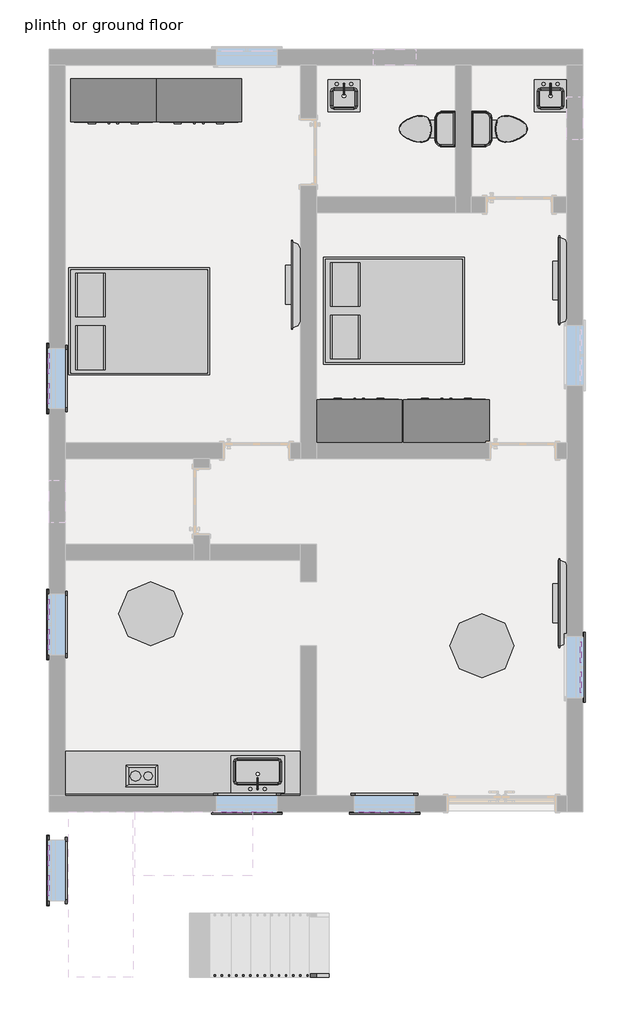
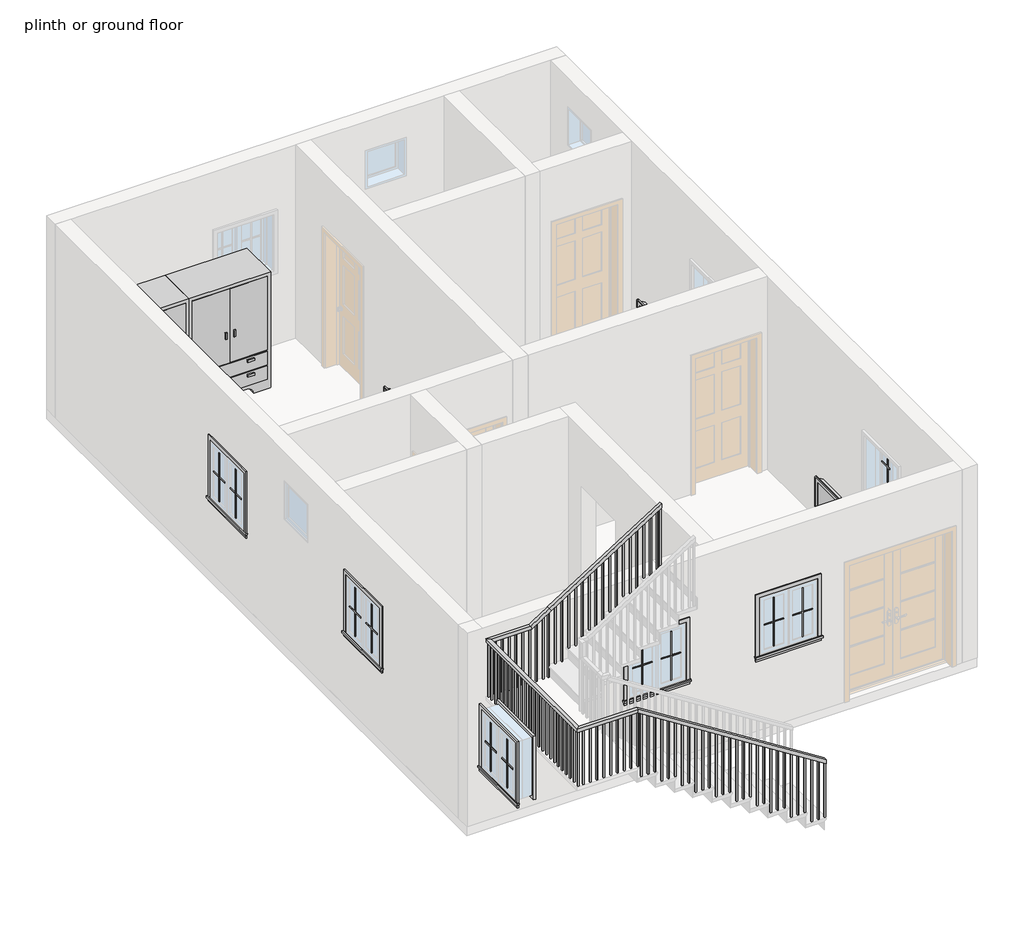
# One storey, part 2 of 3: 24 proxies, 12 furniture elements, 5 flow terminals, 1 railing.
"""IFC4 building model written with IfcOpenShell, lengths in millimetres."""

from ifc_helpers import new_model, si_unit, frame, origin, place, context, project, spatial, polyline, outline, extrude, faceted_brep, transform, mapped, element, save
from components import proxy_fb8a77b2, muntin_pattern_2x2_muntin_pattern_2x2_b3fe6957, muntin_pattern_2x2_muntin_pattern_2x2_3e0ecaf2, trim_window_exterior_flat_with_sill_41619996, trim_window_interior_flat_picture_frame_51c85655, flow_terminal_2ed30f95, flow_terminal_4d548711, toilet_domestic_3d_toilet_domestic_3d_ba6479b0, toilet_domestic_3d_toilet_domestic_3d_30431060, furniture_0315470b, furniture_691b2c5f, furniture_0b81fedb, furniture_ec754799, furniture_52f35bf4, furniture_82e269c4

model = new_model("IFC4")

# Units and contexts
model_context = context("Model", 3, world=origin())
ifc_project = project(units=[si_unit("LENGTHUNIT", "METRE", prefix="MILLI")], contexts=[model_context])

# Site, building, storey
site = spatial("IfcSite", under=ifc_project)
building = spatial("IfcBuilding", under=site)
storey = spatial("IfcBuildingStorey", under=building, Name="plinth or ground floor", Elevation=609.6)

# Proxies
placement = place(None, origin())
proxy_shape = proxy_fb8a77b2(model_context)
element("IfcBuildingElementProxy", 1, Name="Cook Top-2 Unit : 12\" x 18\"", ObjectType="Cook Top-2 Unit : 12\" x 18\"", at=placement, inside=storey, context=model_context, shape_type="MappedRepresentation", body=[
    mapped(proxy_shape, transform((20364.3384757, 6764.8409313, 609.6), x_axis=(0.0, 1.0, 0.0), y_axis=(-1.0, 0.0, 0.0), z_axis=(0.0, 0.0, 1.0))),
])
muntin_pattern_2x2_muntin_pattern_2x2_shape = muntin_pattern_2x2_muntin_pattern_2x2_b3fe6957(model_context)
element("IfcBuildingElementProxy", 2, Name="Muntin Pattern_2x2 : Muntin Pattern_2x2", ObjectType="Muntin Pattern_2x2 : Muntin Pattern_2x2", at=placement, inside=storey, context=model_context, shape_type="MappedRepresentation", body=[
    mapped(muntin_pattern_2x2_muntin_pattern_2x2_shape, transform((19022.8386801, 8785.7284313, 1863.725), x_axis=(0.0, 1.0, 0.0), y_axis=(-1.0, 0.0, 0.0), z_axis=(0.0, 0.0, 1.0))),
])
element("IfcBuildingElementProxy", 3, Name="Muntin Pattern_2x2 : Muntin Pattern_2x2", ObjectType="Muntin Pattern_2x2 : Muntin Pattern_2x2", at=placement, inside=storey, context=model_context, shape_type="MappedRepresentation", body=[
    mapped(muntin_pattern_2x2_muntin_pattern_2x2_shape, transform((19022.8386801, 12290.9284313, 1863.725), x_axis=(0.0, 1.0, 0.0), y_axis=(-1.0, 0.0, 0.0), z_axis=(0.0, 0.0, 1.0))),
])
element("IfcBuildingElementProxy", 4, Name="Muntin Pattern_2x2 : Muntin Pattern_2x2", ObjectType="Muntin Pattern_2x2 : Muntin Pattern_2x2", at=placement, inside=storey, context=model_context, shape_type="MappedRepresentation", body=[
    mapped(muntin_pattern_2x2_muntin_pattern_2x2_shape, transform((26611.0886801, 8604.7534313, 1863.725), x_axis=(0.0, -1.0, 0.0), y_axis=(1.0, 0.0, 0.0), z_axis=(0.0, 0.0, 1.0))),
])
element("IfcBuildingElementProxy", 5, Name="Muntin Pattern_2x2 : Muntin Pattern_2x2", ObjectType="Muntin Pattern_2x2 : Muntin Pattern_2x2", at=placement, inside=storey, context=model_context, shape_type="MappedRepresentation", body=[
    mapped(muntin_pattern_2x2_muntin_pattern_2x2_shape, transform((22047.0261801, 6342.5659313, 1863.725), x_axis=(-1.0, 0.0, 0.0), y_axis=(0.0, -1.0, 0.0), z_axis=(0.0, 0.0, 1.0))),
])
element("IfcBuildingElementProxy", 6, Name="Muntin Pattern_2x2 : Muntin Pattern_2x2", ObjectType="Muntin Pattern_2x2 : Muntin Pattern_2x2", at=placement, inside=storey, context=model_context, shape_type="MappedRepresentation", body=[
    mapped(muntin_pattern_2x2_muntin_pattern_2x2_shape, transform((24009.1761801, 6342.5659313, 1863.725), x_axis=(-1.0, 0.0, 0.0), y_axis=(0.0, -1.0, 0.0), z_axis=(0.0, 0.0, 1.0))),
])
element("IfcBuildingElementProxy", 7, Name="Muntin Pattern_2x2 : Muntin Pattern_2x2", ObjectType="Muntin Pattern_2x2 : Muntin Pattern_2x2", at=placement, inside=storey, context=model_context, shape_type="MappedRepresentation", body=[
    mapped(muntin_pattern_2x2_muntin_pattern_2x2_shape, transform((19022.8386801, 5280.5284313, 1863.725), x_axis=(0.0, 1.0, 0.0), y_axis=(-1.0, 0.0, 0.0), z_axis=(0.0, 0.0, 1.0))),
])
muntin_pattern_2x2_muntin_pattern_2x2_2_shape = muntin_pattern_2x2_muntin_pattern_2x2_3e0ecaf2(model_context)
element("IfcBuildingElementProxy", 8, Name="Muntin Pattern_2x2 : Muntin Pattern_2x2", ObjectType="Muntin Pattern_2x2 : Muntin Pattern_2x2", at=placement, inside=storey, context=model_context, shape_type="MappedRepresentation", body=[
    mapped(muntin_pattern_2x2_muntin_pattern_2x2_2_shape, transform((19022.8386801, 9214.3534313, 1863.725), x_axis=(0.0, -1.0, 0.0), y_axis=(1.0, 0.0, 0.0), z_axis=(0.0, 0.0, 1.0))),
])
element("IfcBuildingElementProxy", 9, Name="Muntin Pattern_2x2 : Muntin Pattern_2x2", ObjectType="Muntin Pattern_2x2 : Muntin Pattern_2x2", at=placement, inside=storey, context=model_context, shape_type="MappedRepresentation", body=[
    mapped(muntin_pattern_2x2_muntin_pattern_2x2_2_shape, transform((19022.8386801, 12719.5534313, 1863.725), x_axis=(0.0, -1.0, 0.0), y_axis=(1.0, 0.0, 0.0), z_axis=(0.0, 0.0, 1.0))),
])
element("IfcBuildingElementProxy", 10, Name="Muntin Pattern_2x2 : Muntin Pattern_2x2", ObjectType="Muntin Pattern_2x2 : Muntin Pattern_2x2", at=placement, inside=storey, context=model_context, shape_type="MappedRepresentation", body=[
    mapped(muntin_pattern_2x2_muntin_pattern_2x2_2_shape, transform((26611.0886801, 8176.1284313, 1863.725), x_axis=(0.0, 1.0, 0.0), y_axis=(-1.0, 0.0, 0.0), z_axis=(0.0, 0.0, 1.0))),
])
element("IfcBuildingElementProxy", 11, Name="Muntin Pattern_2x2 : Muntin Pattern_2x2", ObjectType="Muntin Pattern_2x2 : Muntin Pattern_2x2", at=placement, inside=storey, context=model_context, shape_type="MappedRepresentation", body=[
    mapped(muntin_pattern_2x2_muntin_pattern_2x2_2_shape, transform((21618.4011801, 6342.5659313, 1863.725), x_axis=(1.0, 0.0, 0.0), y_axis=(0.0, 1.0, 0.0), z_axis=(0.0, 0.0, 1.0))),
])
element("IfcBuildingElementProxy", 12, Name="Muntin Pattern_2x2 : Muntin Pattern_2x2", ObjectType="Muntin Pattern_2x2 : Muntin Pattern_2x2", at=placement, inside=storey, context=model_context, shape_type="MappedRepresentation", body=[
    mapped(muntin_pattern_2x2_muntin_pattern_2x2_2_shape, transform((23580.5511801, 6342.5659313, 1863.725), x_axis=(1.0, 0.0, 0.0), y_axis=(0.0, 1.0, 0.0), z_axis=(0.0, 0.0, 1.0))),
])
element("IfcBuildingElementProxy", 13, Name="Muntin Pattern_2x2 : Muntin Pattern_2x2", ObjectType="Muntin Pattern_2x2 : Muntin Pattern_2x2", at=placement, inside=storey, context=model_context, shape_type="MappedRepresentation", body=[
    mapped(muntin_pattern_2x2_muntin_pattern_2x2_2_shape, transform((19022.8386801, 5709.1534313, 1863.725), x_axis=(0.0, -1.0, 0.0), y_axis=(1.0, 0.0, 0.0), z_axis=(0.0, 0.0, 1.0))),
])
trim_window_exterior_flat_with_sill_shape = trim_window_exterior_flat_with_sill_41619996(model_context)
element("IfcBuildingElementProxy", 14, Name="Trim-Window-Exterior-Flat : with Sill", ObjectType="Trim-Window-Exterior-Flat : with Sill", at=placement, inside=storey, context=model_context, shape_type="MappedRepresentation", body=[
    mapped(trim_window_exterior_flat_with_sill_shape, transform((19013.3136801, 9000.0409313, 2708.275), x_axis=(0.0, -1.0, 0.0), y_axis=(0.0, 0.0, 1.0), z_axis=(-1.0, 0.0, 0.0))),
])
element("IfcBuildingElementProxy", 15, Name="Trim-Window-Exterior-Flat : with Sill", ObjectType="Trim-Window-Exterior-Flat : with Sill", at=placement, inside=storey, context=model_context, shape_type="MappedRepresentation", body=[
    mapped(trim_window_exterior_flat_with_sill_shape, transform((19013.3136801, 12505.2409313, 2708.275), x_axis=(0.0, -1.0, 0.0), y_axis=(0.0, 0.0, 1.0), z_axis=(-1.0, 0.0, 0.0))),
])
element("IfcBuildingElementProxy", 16, Name="Trim-Window-Exterior-Flat : with Sill", ObjectType="Trim-Window-Exterior-Flat : with Sill", at=placement, inside=storey, context=model_context, shape_type="MappedRepresentation", body=[
    mapped(trim_window_exterior_flat_with_sill_shape, transform((26620.6136801, 8390.4409313, 2708.275), x_axis=(0.0, 1.0, 0.0), y_axis=(0.0, 0.0, 1.0), z_axis=(1.0, 0.0, 0.0))),
])
element("IfcBuildingElementProxy", 17, Name="Trim-Window-Exterior-Flat : with Sill", ObjectType="Trim-Window-Exterior-Flat : with Sill", at=placement, inside=storey, context=model_context, shape_type="MappedRepresentation", body=[
    mapped(trim_window_exterior_flat_with_sill_shape, transform((21832.7136801, 6333.0409313, 2708.275), x_axis=(1.0, 0.0, 0.0), y_axis=(0.0, 0.0, 1.0), z_axis=(0.0, -1.0, 0.0))),
])
element("IfcBuildingElementProxy", 18, Name="Trim-Window-Exterior-Flat : with Sill", ObjectType="Trim-Window-Exterior-Flat : with Sill", at=placement, inside=storey, context=model_context, shape_type="MappedRepresentation", body=[
    mapped(trim_window_exterior_flat_with_sill_shape, transform((23794.8636801, 6333.0409313, 2708.275), x_axis=(1.0, 0.0, 0.0), y_axis=(0.0, 0.0, 1.0), z_axis=(0.0, -1.0, 0.0))),
])
element("IfcBuildingElementProxy", 19, Name="Trim-Window-Exterior-Flat : with Sill", ObjectType="Trim-Window-Exterior-Flat : with Sill", at=placement, inside=storey, context=model_context, shape_type="MappedRepresentation", body=[
    mapped(trim_window_exterior_flat_with_sill_shape, transform((19013.3136801, 5494.8409313, 2708.275), x_axis=(0.0, -1.0, 0.0), y_axis=(0.0, 0.0, 1.0), z_axis=(-1.0, 0.0, 0.0))),
])
trim_window_interior_flat_picture_frame_shape = trim_window_interior_flat_picture_frame_51c85655(model_context)
element("IfcBuildingElementProxy", 20, Name="Trim-Window-Interior-Flat : Picture Frame", ObjectType="Trim-Window-Interior-Flat : Picture Frame", at=placement, inside=storey, context=model_context, shape_type="MappedRepresentation", body=[
    mapped(trim_window_interior_flat_picture_frame_shape, transform((19241.9136801, 9000.0409313, 2708.275), x_axis=(0.0, 1.0, 0.0), y_axis=(0.0, 0.0, 1.0), z_axis=(1.0, 0.0, 0.0))),
])
element("IfcBuildingElementProxy", 21, Name="Trim-Window-Interior-Flat : Picture Frame", ObjectType="Trim-Window-Interior-Flat : Picture Frame", at=placement, inside=storey, context=model_context, shape_type="MappedRepresentation", body=[
    mapped(trim_window_interior_flat_picture_frame_shape, transform((19241.9136801, 12505.2409313, 2708.275), x_axis=(0.0, 1.0, 0.0), y_axis=(0.0, 0.0, 1.0), z_axis=(1.0, 0.0, 0.0))),
])
element("IfcBuildingElementProxy", 22, Name="Trim-Window-Interior-Flat : Picture Frame", ObjectType="Trim-Window-Interior-Flat : Picture Frame", at=placement, inside=storey, context=model_context, shape_type="MappedRepresentation", body=[
    mapped(trim_window_interior_flat_picture_frame_shape, transform((21832.7136801, 6561.6409313, 2708.275), x_axis=(-1.0, 0.0, 0.0), y_axis=(0.0, 0.0, 1.0), z_axis=(0.0, 1.0, 0.0))),
])
element("IfcBuildingElementProxy", 23, Name="Trim-Window-Interior-Flat : Picture Frame", ObjectType="Trim-Window-Interior-Flat : Picture Frame", at=placement, inside=storey, context=model_context, shape_type="MappedRepresentation", body=[
    mapped(trim_window_interior_flat_picture_frame_shape, transform((23794.8636801, 6561.6409313, 2708.275), x_axis=(-1.0, 0.0, 0.0), y_axis=(0.0, 0.0, 1.0), z_axis=(0.0, 1.0, 0.0))),
])
element("IfcBuildingElementProxy", 24, Name="Trim-Window-Interior-Flat : Picture Frame", ObjectType="Trim-Window-Interior-Flat : Picture Frame", at=placement, inside=storey, context=model_context, shape_type="MappedRepresentation", body=[
    mapped(trim_window_interior_flat_picture_frame_shape, transform((19241.9136801, 5494.8409313, 2708.275), x_axis=(0.0, 1.0, 0.0), y_axis=(0.0, 0.0, 1.0), z_axis=(1.0, 0.0, 0.0))),
])

# Flow terminals
flow_terminal_shape = flow_terminal_2ed30f95(model_context)
element("IfcFlowTerminal", 25, ObjectType="Sink Kitchen-Island : 18\" x 18\"", at=placement, inside=storey, context=model_context, shape_type="MappedRepresentation", body=[
    mapped(flow_terminal_shape, transform((23201.3244395, 16528.7955302, 609.6), x_axis=(1.0, 0.0, 0.0), y_axis=(0.0, 1.0, 0.0), z_axis=(0.0, 0.0, 1.0))),
])
element("IfcFlowTerminal", 26, ObjectType="Sink Kitchen-Island : 18\" x 18\"", at=placement, inside=storey, context=model_context, shape_type="MappedRepresentation", body=[
    mapped(flow_terminal_shape, transform((26147.7244395, 16528.7955302, 609.6), x_axis=(1.0, 0.0, 0.0), y_axis=(0.0, 1.0, 0.0), z_axis=(0.0, 0.0, 1.0))),
])
flow_terminal_2_shape = flow_terminal_4d548711(model_context)
element("IfcFlowTerminal", 27, ObjectType="Sink Kitchen-Single : 30\" x 21\"", at=placement, inside=storey, context=model_context, shape_type="MappedRepresentation", body=[
    mapped(flow_terminal_2_shape, transform((22000.8029206, 6868.7863324, 609.6), x_axis=(-1.0, 0.0, 0.0), y_axis=(0.0, -1.0, 0.0), z_axis=(0.0, 0.0, 1.0))),
])
toilet_domestic_3d_toilet_domestic_3d_shape = toilet_domestic_3d_toilet_domestic_3d_ba6479b0(model_context)
toilet_domestic_3d_toilet_domestic_3d_2_shape = toilet_domestic_3d_toilet_domestic_3d_30431060(model_context)
element("IfcFlowTerminal", 28, ObjectType="Toilet-Domestic-3D : Toilet-Domestic-3D", at=placement, inside=storey, context=model_context, shape_type="MappedRepresentation", body=[
    mapped(toilet_domestic_3d_toilet_domestic_3d_shape, transform((24309.8176527, 16061.2409313, 609.6), x_axis=(0.0, -1.0, 0.0), y_axis=(1.0, 0.0, 0.0), z_axis=(0.0, 0.0, 1.0))),
    mapped(toilet_domestic_3d_toilet_domestic_3d_2_shape, transform((24309.8176527, 16061.2409313, 609.6), x_axis=(0.0, -1.0, 0.0), y_axis=(1.0, 0.0, 0.0), z_axis=(0.0, 0.0, 1.0))),
])
element("IfcFlowTerminal", 29, ObjectType="Toilet-Domestic-3D : Toilet-Domestic-3D", at=placement, inside=storey, context=model_context, shape_type="MappedRepresentation", body=[
    mapped(toilet_domestic_3d_toilet_domestic_3d_shape, transform((25527.8097074, 16061.2409313, 609.6), x_axis=(0.0, 1.0, 0.0), y_axis=(-1.0, 0.0, 0.0), z_axis=(0.0, 0.0, 1.0))),
    mapped(toilet_domestic_3d_toilet_domestic_3d_2_shape, transform((25527.8097074, 16061.2409313, 609.6), x_axis=(0.0, 1.0, 0.0), y_axis=(-1.0, 0.0, 0.0), z_axis=(0.0, 0.0, 1.0))),
])

# Furniture
furniture_shape = furniture_0315470b(model_context)
element("IfcFurniture", 30, ObjectType="Bed-Box : Queen 60\" x 79\"", at=placement, inside=storey, context=model_context, shape_type="MappedRepresentation", body=[
    mapped(furniture_shape, transform((20061.5841719, 12978.8884723, 609.6), x_axis=(0.0, 1.0, 0.0), y_axis=(-1.0, 0.0, 0.0), z_axis=(0.0, 0.0, 1.0))),
])
element("IfcFurniture", 31, ObjectType="Bed-Box : Queen 60\" x 79\"", at=placement, inside=storey, context=model_context, shape_type="MappedRepresentation", body=[
    mapped(furniture_shape, transform((23693.7841719, 13131.2884723, 609.6), x_axis=(0.0, 1.0, 0.0), y_axis=(-1.0, 0.0, 0.0), z_axis=(0.0, 0.0, 1.0))),
])
furniture_2_shape = furniture_691b2c5f(model_context)
element("IfcFurniture", 32, ObjectType="Counter Top w Sink Hole : 24\" Depth", at=placement, inside=storey, context=model_context, shape_type="MappedRepresentation", body=[
    mapped(furniture_2_shape, transform((21394.251385, 6561.6409313, 609.6), x_axis=(-1.0, 0.0, 0.0), y_axis=(0.0, -1.0, 0.0), z_axis=(0.0, 0.0, 1.0))),
])
furniture_3_shape = furniture_0b81fedb(model_context)
element("IfcFurniture", 33, ObjectType="TV - Flat Screen : 50\"", at=placement, inside=storey, context=model_context, shape_type="MappedRepresentation", body=[
    mapped(furniture_3_shape, transform((26346.1750564, 9300.8964171, 609.6), x_axis=(0.0, -1.0, 0.0), y_axis=(1.0, 0.0, 0.0), z_axis=(0.0, 0.0, 1.0))),
])
element("IfcFurniture", 34, ObjectType="TV - Flat Screen : 50\"", at=placement, inside=storey, context=model_context, shape_type="MappedRepresentation", body=[
    mapped(furniture_3_shape, transform((26346.1750564, 13898.2964171, 609.6), x_axis=(0.0, -1.0, 0.0), y_axis=(1.0, 0.0, 0.0), z_axis=(0.0, 0.0, 1.0))),
])
element("IfcFurniture", 35, ObjectType="TV - Flat Screen : 50\"", at=placement, inside=storey, context=model_context, shape_type="MappedRepresentation", body=[
    mapped(furniture_3_shape, transform((22536.1750564, 13834.7964171, 609.6), x_axis=(0.0, -1.0, 0.0), y_axis=(1.0, 0.0, 0.0), z_axis=(0.0, 0.0, 1.0))),
])
furniture_4_shape = furniture_ec754799(model_context)
element("IfcFurniture", 36, ObjectType="Table-Dining Round : 36\" Diameter", at=placement, inside=storey, context=model_context, shape_type="MappedRepresentation", body=[
    mapped(furniture_4_shape, transform((25081.8317129, 8880.1196198, 609.6), x_axis=(1.0, 0.0, 0.0), y_axis=(0.0, 1.0, 0.0), z_axis=(0.0, 0.0, 1.0))),
])
furniture_5_shape = furniture_52f35bf4(model_context)
element("IfcFurniture", 37, ObjectType="Table-Dining Round w Chairs : 36\" Diameter", at=placement, inside=storey, context=model_context, shape_type="MappedRepresentation", body=[
    mapped(furniture_5_shape, transform((20357.4317129, 9337.3196198, 609.6), x_axis=(1.0, 0.0, 0.0), y_axis=(0.0, 1.0, 0.0), z_axis=(0.0, 0.0, 1.0))),
])
furniture_6_shape = furniture_82e269c4(model_context)
element("IfcFurniture", 38, ObjectType="Wardrobe : 48\" x 72\" x 24\"", at=placement, inside=storey, context=model_context, shape_type="MappedRepresentation", body=[
    mapped(furniture_6_shape, transform((23163.7204202, 11311.9021217, 609.6), x_axis=(-1.0, 0.0, 0.0), y_axis=(0.0, -1.0, 0.0), z_axis=(0.0, 0.0, 1.0))),
])
element("IfcFurniture", 39, ObjectType="Wardrobe : 48\" x 72\" x 24\"", at=placement, inside=storey, context=model_context, shape_type="MappedRepresentation", body=[
    mapped(furniture_6_shape, transform((20196.9069399, 17051.3797408, 609.6), x_axis=(1.0, 0.0, 0.0), y_axis=(0.0, 1.0, 0.0), z_axis=(0.0, 0.0, 1.0))),
])
element("IfcFurniture", 40, ObjectType="Wardrobe : 48\" x 72\" x 24\"", at=placement, inside=storey, context=model_context, shape_type="MappedRepresentation", body=[
    mapped(furniture_6_shape, transform((21416.1069399, 17051.3797408, 609.6), x_axis=(1.0, 0.0, 0.0), y_axis=(0.0, 1.0, 0.0), z_axis=(0.0, 0.0, 1.0))),
])
element("IfcFurniture", 41, ObjectType="Wardrobe : 48\" x 72\" x 24\"", at=placement, inside=storey, context=model_context, shape_type="MappedRepresentation", body=[
    mapped(furniture_6_shape, transform((24408.3204202, 11311.9021217, 609.6), x_axis=(-1.0, 0.0, 0.0), y_axis=(0.0, -1.0, 0.0), z_axis=(0.0, 0.0, 1.0))),
])

# Railing
element("IfcRailing", 42, ObjectType="Handrail - Rectangular", at=placement, inside=storey, context=model_context, shape_type="SolidModel", body=[
    faceted_brep([(23001.1136801, 3970.8409313, 1701.8), (23001.1136801, 3970.8409313, 1641.586276), (23001.1136801, 4021.6409313, 1641.586276), (23001.1136801, 4021.6409313, 1701.8), (20207.1136801, 3970.8409313, 3479.8), (20192.3206852, 3970.8409313, 3429.0), (20192.3206852, 4021.6409313, 3429.0), (20207.1136801, 4021.6409313, 3479.8), (19292.7136801, 3970.8409313, 3479.8), (19292.7136801, 3970.8409313, 3429.0), (19343.5136801, 4021.6409313, 3429.0), (19343.5136801, 4021.6409313, 3479.8), (19292.7136801, 6333.0409313, 3479.8), (19292.7136801, 6333.0409313, 3429.0), (19343.5136801, 6282.2409313, 3429.0), (19343.5136801, 6282.2409313, 3479.8), (19927.7136801, 6333.0409313, 3479.8), (19942.506675, 6333.0409313, 3429.0), (19942.506675, 6282.2409313, 3429.0), (19927.7136801, 6282.2409313, 3479.8), (20207.1136801, 6333.0409313, 3657.6), (20234.3869551, 6333.0409313, 3614.7419964), (20234.3869551, 6282.2409313, 3614.7419964), (20207.1136801, 6282.2409313, 3657.6), (21883.5136801, 6333.0409313, 4724.4), (21883.5136801, 6282.2409313, 4724.4), (21883.5136801, 6282.2409313, 4664.186276), (21883.5136801, 6333.0409313, 4664.186276)], [[[0, 1, 2, 3]], [[1, 0, 4, 5]], [[2, 1, 5, 6]], [[3, 2, 6, 7]], [[0, 3, 7, 4]], [[5, 4, 8, 9]], [[6, 5, 9, 10]], [[7, 6, 10, 11]], [[4, 7, 11, 8]], [[9, 8, 12, 13]], [[10, 9, 13, 14]], [[11, 10, 14, 15]], [[8, 11, 15, 12]], [[13, 12, 16, 17]], [[14, 13, 17, 18]], [[15, 14, 18, 19]], [[12, 15, 19, 16]], [[17, 16, 20, 21]], [[18, 17, 21, 22]], [[19, 18, 22, 23]], [[16, 19, 23, 20]], [[24, 25, 26, 27]], [[21, 20, 24, 27]], [[22, 21, 27, 26]], [[23, 22, 26, 25]], [[20, 23, 25, 24]]]),
    extrude(outline(polyline([(4625.7976396, 21823.1886801), (3632.2, 21823.1886801), (3632.2, 21842.2386801), (4637.9203669, 21842.2386801), (4625.7976396, 21823.1886801)])), frame((0.0, 6298.1159313, 0.0), z_axis=(0.0, 1.0, 0.0), x_axis=(0.0, 0.0, 1.0)), (0.0, 0.0, 1.0), 19.05),
    extrude(outline(polyline([(4561.1430941, 21721.5886801), (3632.2, 21721.5886801), (3632.2, 21740.6386801), (4573.2658214, 21740.6386801), (4561.1430941, 21721.5886801)])), frame((0.0, 6298.1159313, 0.0), z_axis=(0.0, 1.0, 0.0), x_axis=(0.0, 0.0, 1.0)), (0.0, 0.0, 1.0), 19.05),
    extrude(outline(polyline([(4496.4885487, 21619.9886801), (3632.2, 21619.9886801), (3632.2, 21639.0386801), (4508.611276, 21639.0386801), (4496.4885487, 21619.9886801)])), frame((0.0, 6298.1159313, 0.0), z_axis=(0.0, 1.0, 0.0), x_axis=(0.0, 0.0, 1.0)), (0.0, 0.0, 1.0), 19.05),
    extrude(outline(polyline([(4431.8340032, 21518.3886801), (3454.4, 21518.3886801), (3454.4, 21537.4386801), (4443.9567305, 21537.4386801), (4431.8340032, 21518.3886801)])), frame((0.0, 6298.1159313, 0.0), z_axis=(0.0, 1.0, 0.0), x_axis=(0.0, 0.0, 1.0)), (0.0, 0.0, 1.0), 19.05),
    extrude(outline(polyline([(4367.1794578, 21416.7886801), (3454.4, 21416.7886801), (3454.4, 21435.8386801), (4379.3021851, 21435.8386801), (4367.1794578, 21416.7886801)])), frame((0.0, 6298.1159313, 0.0), z_axis=(0.0, 1.0, 0.0), x_axis=(0.0, 0.0, 1.0)), (0.0, 0.0, 1.0), 19.05),
    extrude(outline(polyline([(4302.5249123, 21315.1886801), (3454.4, 21315.1886801), (3454.4, 21334.2386801), (4314.6476396, 21334.2386801), (4302.5249123, 21315.1886801)])), frame((0.0, 6298.1159313, 0.0), z_axis=(0.0, 1.0, 0.0), x_axis=(0.0, 0.0, 1.0)), (0.0, 0.0, 1.0), 19.05),
    extrude(outline(polyline([(4237.8703669, 21213.5886801), (3276.6, 21213.5886801), (3276.6, 21232.6386801), (4249.9930941, 21232.6386801), (4237.8703669, 21213.5886801)])), frame((0.0, 6298.1159313, 0.0), z_axis=(0.0, 1.0, 0.0), x_axis=(0.0, 0.0, 1.0)), (0.0, 0.0, 1.0), 19.05),
    extrude(outline(polyline([(4173.2158214, 21111.9886801), (3276.6, 21111.9886801), (3276.6, 21131.0386801), (4185.3385487, 21131.0386801), (4173.2158214, 21111.9886801)])), frame((0.0, 6298.1159313, 0.0), z_axis=(0.0, 1.0, 0.0), x_axis=(0.0, 0.0, 1.0)), (0.0, 0.0, 1.0), 19.05),
    extrude(outline(polyline([(4108.561276, 21010.3886801), (3098.8, 21010.3886801), (3098.8, 21029.4386801), (4120.6840032, 21029.4386801), (4108.561276, 21010.3886801)])), frame((0.0, 6298.1159313, 0.0), z_axis=(0.0, 1.0, 0.0), x_axis=(0.0, 0.0, 1.0)), (0.0, 0.0, 1.0), 19.05),
    extrude(outline(polyline([(4043.9067305, 20908.7886801), (3098.8, 20908.7886801), (3098.8, 20927.8386801), (4056.0294578, 20927.8386801), (4043.9067305, 20908.7886801)])), frame((0.0, 6298.1159313, 0.0), z_axis=(0.0, 1.0, 0.0), x_axis=(0.0, 0.0, 1.0)), (0.0, 0.0, 1.0), 19.05),
    extrude(outline(polyline([(3979.2521851, 20807.1886801), (3098.8, 20807.1886801), (3098.8, 20826.2386801), (3991.3749123, 20826.2386801), (3979.2521851, 20807.1886801)])), frame((0.0, 6298.1159313, 0.0), z_axis=(0.0, 1.0, 0.0), x_axis=(0.0, 0.0, 1.0)), (0.0, 0.0, 1.0), 19.05),
    extrude(outline(polyline([(3914.5976396, 20705.5886801), (2921.0, 20705.5886801), (2921.0, 20724.6386801), (3926.7203669, 20724.6386801), (3914.5976396, 20705.5886801)])), frame((0.0, 6298.1159313, 0.0), z_axis=(0.0, 1.0, 0.0), x_axis=(0.0, 0.0, 1.0)), (0.0, 0.0, 1.0), 19.05),
    extrude(outline(polyline([(3849.9430941, 20603.9886801), (2921.0, 20603.9886801), (2921.0, 20623.0386801), (3862.0658214, 20623.0386801), (3849.9430941, 20603.9886801)])), frame((0.0, 6298.1159313, 0.0), z_axis=(0.0, 1.0, 0.0), x_axis=(0.0, 0.0, 1.0)), (0.0, 0.0, 1.0), 19.05),
    extrude(outline(polyline([(3785.2885487, 20502.3886801), (2921.0, 20502.3886801), (2921.0, 20521.4386801), (3797.411276, 20521.4386801), (3785.2885487, 20502.3886801)])), frame((0.0, 6298.1159313, 0.0), z_axis=(0.0, 1.0, 0.0), x_axis=(0.0, 0.0, 1.0)), (0.0, 0.0, 1.0), 19.05),
    extrude(outline(polyline([(3720.6340032, 20400.7886801), (2743.2, 20400.7886801), (2743.2, 20419.8386801), (3732.7567305, 20419.8386801), (3720.6340032, 20400.7886801)])), frame((0.0, 6298.1159313, 0.0), z_axis=(0.0, 1.0, 0.0), x_axis=(0.0, 0.0, 1.0)), (0.0, 0.0, 1.0), 19.05),
    extrude(outline(polyline([(3655.9794578, 20299.1886801), (2743.2, 20299.1886801), (2743.2, 20318.2386801), (3668.1021851, 20318.2386801), (3655.9794578, 20299.1886801)])), frame((0.0, 6298.1159313, 0.0), z_axis=(0.0, 1.0, 0.0), x_axis=(0.0, 0.0, 1.0)), (0.0, 0.0, 1.0), 19.05),
    extrude(outline(polyline([(3542.8340032, 20121.3886801), (2565.4, 20121.3886801), (2565.4, 20140.4386801), (3554.9567305, 20140.4386801), (3542.8340032, 20121.3886801)])), frame((0.0, 6298.1159313, 0.0), z_axis=(0.0, 1.0, 0.0), x_axis=(0.0, 0.0, 1.0)), (0.0, 0.0, 1.0), 19.05),
    extrude(outline(polyline([(3478.1794578, 20019.7886801), (2565.4, 20019.7886801), (2565.4, 20038.8386801), (3490.3021851, 20038.8386801), (3478.1794578, 20019.7886801)])), frame((0.0, 6298.1159313, 0.0), z_axis=(0.0, 1.0, 0.0), x_axis=(0.0, 0.0, 1.0)), (0.0, 0.0, 1.0), 19.05),
    extrude(outline(polyline([(19918.1886801, 6317.1659313), (19937.2386801, 6317.1659313), (19937.2386801, 6298.1159313), (19918.1886801, 6298.1159313), (19918.1886801, 6317.1659313)])), frame((0.0, 0.0, 2565.4), z_axis=(0.0, 0.0, 1.0), x_axis=(1.0, 0.0, 0.0)), (0.0, 0.0, 1.0), 863.6),
    extrude(outline(polyline([(19816.5886801, 6317.1659313), (19835.6386801, 6317.1659313), (19835.6386801, 6298.1159313), (19816.5886801, 6298.1159313), (19816.5886801, 6317.1659313)])), frame((0.0, 0.0, 2565.4), z_axis=(0.0, 0.0, 1.0), x_axis=(1.0, 0.0, 0.0)), (0.0, 0.0, 1.0), 863.6),
    extrude(outline(polyline([(19714.9886801, 6317.1659313), (19734.0386801, 6317.1659313), (19734.0386801, 6298.1159313), (19714.9886801, 6298.1159313), (19714.9886801, 6317.1659313)])), frame((0.0, 0.0, 2565.4), z_axis=(0.0, 0.0, 1.0), x_axis=(1.0, 0.0, 0.0)), (0.0, 0.0, 1.0), 863.6),
    extrude(outline(polyline([(19613.3886801, 6317.1659313), (19632.4386801, 6317.1659313), (19632.4386801, 6298.1159313), (19613.3886801, 6298.1159313), (19613.3886801, 6317.1659313)])), frame((0.0, 0.0, 2565.4), z_axis=(0.0, 0.0, 1.0), x_axis=(1.0, 0.0, 0.0)), (0.0, 0.0, 1.0), 863.6),
    extrude(outline(polyline([(19511.7886801, 6317.1659313), (19530.8386801, 6317.1659313), (19530.8386801, 6298.1159313), (19511.7886801, 6298.1159313), (19511.7886801, 6317.1659313)])), frame((0.0, 0.0, 2565.4), z_axis=(0.0, 0.0, 1.0), x_axis=(1.0, 0.0, 0.0)), (0.0, 0.0, 1.0), 863.6),
    extrude(outline(polyline([(19410.1886801, 6317.1659313), (19429.2386801, 6317.1659313), (19429.2386801, 6298.1159313), (19410.1886801, 6298.1159313), (19410.1886801, 6317.1659313)])), frame((0.0, 0.0, 2565.4), z_axis=(0.0, 0.0, 1.0), x_axis=(1.0, 0.0, 0.0)), (0.0, 0.0, 1.0), 863.6),
    extrude(outline(polyline([(19308.5886801, 6221.9159313), (19308.5886801, 6240.9659313), (19327.6386801, 6240.9659313), (19327.6386801, 6221.9159313), (19308.5886801, 6221.9159313)])), frame((0.0, 0.0, 2565.4), z_axis=(0.0, 0.0, 1.0), x_axis=(1.0, 0.0, 0.0)), (0.0, 0.0, 1.0), 863.6),
    extrude(outline(polyline([(19308.5886801, 6120.3159313), (19308.5886801, 6139.3659313), (19327.6386801, 6139.3659313), (19327.6386801, 6120.3159313), (19308.5886801, 6120.3159313)])), frame((0.0, 0.0, 2565.4), z_axis=(0.0, 0.0, 1.0), x_axis=(1.0, 0.0, 0.0)), (0.0, 0.0, 1.0), 863.6),
    extrude(outline(polyline([(19308.5886801, 6018.7159313), (19308.5886801, 6037.7659313), (19327.6386801, 6037.7659313), (19327.6386801, 6018.7159313), (19308.5886801, 6018.7159313)])), frame((0.0, 0.0, 2565.4), z_axis=(0.0, 0.0, 1.0), x_axis=(1.0, 0.0, 0.0)), (0.0, 0.0, 1.0), 863.6),
    extrude(outline(polyline([(19308.5886801, 5917.1159313), (19308.5886801, 5936.1659313), (19327.6386801, 5936.1659313), (19327.6386801, 5917.1159313), (19308.5886801, 5917.1159313)])), frame((0.0, 0.0, 2565.4), z_axis=(0.0, 0.0, 1.0), x_axis=(1.0, 0.0, 0.0)), (0.0, 0.0, 1.0), 863.6),
    extrude(outline(polyline([(19308.5886801, 5815.5159313), (19308.5886801, 5834.5659313), (19327.6386801, 5834.5659313), (19327.6386801, 5815.5159313), (19308.5886801, 5815.5159313)])), frame((0.0, 0.0, 2565.4), z_axis=(0.0, 0.0, 1.0), x_axis=(1.0, 0.0, 0.0)), (0.0, 0.0, 1.0), 863.6),
    extrude(outline(polyline([(19308.5886801, 5713.9159313), (19308.5886801, 5732.9659313), (19327.6386801, 5732.9659313), (19327.6386801, 5713.9159313), (19308.5886801, 5713.9159313)])), frame((0.0, 0.0, 2565.4), z_axis=(0.0, 0.0, 1.0), x_axis=(1.0, 0.0, 0.0)), (0.0, 0.0, 1.0), 863.6),
    extrude(outline(polyline([(19308.5886801, 5612.3159313), (19308.5886801, 5631.3659313), (19327.6386801, 5631.3659313), (19327.6386801, 5612.3159313), (19308.5886801, 5612.3159313)])), frame((0.0, 0.0, 2565.4), z_axis=(0.0, 0.0, 1.0), x_axis=(1.0, 0.0, 0.0)), (0.0, 0.0, 1.0), 863.6),
    extrude(outline(polyline([(19308.5886801, 5510.7159313), (19308.5886801, 5529.7659313), (19327.6386801, 5529.7659313), (19327.6386801, 5510.7159313), (19308.5886801, 5510.7159313)])), frame((0.0, 0.0, 2565.4), z_axis=(0.0, 0.0, 1.0), x_axis=(1.0, 0.0, 0.0)), (0.0, 0.0, 1.0), 863.6),
    extrude(outline(polyline([(19308.5886801, 5409.1159313), (19308.5886801, 5428.1659313), (19327.6386801, 5428.1659313), (19327.6386801, 5409.1159313), (19308.5886801, 5409.1159313)])), frame((0.0, 0.0, 2565.4), z_axis=(0.0, 0.0, 1.0), x_axis=(1.0, 0.0, 0.0)), (0.0, 0.0, 1.0), 863.6),
    extrude(outline(polyline([(19308.5886801, 5307.5159313), (19308.5886801, 5326.5659313), (19327.6386801, 5326.5659313), (19327.6386801, 5307.5159313), (19308.5886801, 5307.5159313)])), frame((0.0, 0.0, 2565.4), z_axis=(0.0, 0.0, 1.0), x_axis=(1.0, 0.0, 0.0)), (0.0, 0.0, 1.0), 863.6),
    extrude(outline(polyline([(19308.5886801, 5205.9159313), (19308.5886801, 5224.9659313), (19327.6386801, 5224.9659313), (19327.6386801, 5205.9159313), (19308.5886801, 5205.9159313)])), frame((0.0, 0.0, 2565.4), z_axis=(0.0, 0.0, 1.0), x_axis=(1.0, 0.0, 0.0)), (0.0, 0.0, 1.0), 863.6),
    extrude(outline(polyline([(19308.5886801, 5104.3159313), (19308.5886801, 5123.3659313), (19327.6386801, 5123.3659313), (19327.6386801, 5104.3159313), (19308.5886801, 5104.3159313)])), frame((0.0, 0.0, 2565.4), z_axis=(0.0, 0.0, 1.0), x_axis=(1.0, 0.0, 0.0)), (0.0, 0.0, 1.0), 863.6),
    extrude(outline(polyline([(19308.5886801, 5002.7159313), (19308.5886801, 5021.7659313), (19327.6386801, 5021.7659313), (19327.6386801, 5002.7159313), (19308.5886801, 5002.7159313)])), frame((0.0, 0.0, 2565.4), z_axis=(0.0, 0.0, 1.0), x_axis=(1.0, 0.0, 0.0)), (0.0, 0.0, 1.0), 863.6),
    extrude(outline(polyline([(19308.5886801, 4901.1159313), (19308.5886801, 4920.1659313), (19327.6386801, 4920.1659313), (19327.6386801, 4901.1159313), (19308.5886801, 4901.1159313)])), frame((0.0, 0.0, 2565.4), z_axis=(0.0, 0.0, 1.0), x_axis=(1.0, 0.0, 0.0)), (0.0, 0.0, 1.0), 863.6),
    extrude(outline(polyline([(19308.5886801, 4799.5159313), (19308.5886801, 4818.5659313), (19327.6386801, 4818.5659313), (19327.6386801, 4799.5159313), (19308.5886801, 4799.5159313)])), frame((0.0, 0.0, 2565.4), z_axis=(0.0, 0.0, 1.0), x_axis=(1.0, 0.0, 0.0)), (0.0, 0.0, 1.0), 863.6),
    extrude(outline(polyline([(19308.5886801, 4697.9159313), (19308.5886801, 4716.9659313), (19327.6386801, 4716.9659313), (19327.6386801, 4697.9159313), (19308.5886801, 4697.9159313)])), frame((0.0, 0.0, 2565.4), z_axis=(0.0, 0.0, 1.0), x_axis=(1.0, 0.0, 0.0)), (0.0, 0.0, 1.0), 863.6),
    extrude(outline(polyline([(19308.5886801, 4596.3159313), (19308.5886801, 4615.3659313), (19327.6386801, 4615.3659313), (19327.6386801, 4596.3159313), (19308.5886801, 4596.3159313)])), frame((0.0, 0.0, 2565.4), z_axis=(0.0, 0.0, 1.0), x_axis=(1.0, 0.0, 0.0)), (0.0, 0.0, 1.0), 863.6),
    extrude(outline(polyline([(19308.5886801, 4494.7159313), (19308.5886801, 4513.7659313), (19327.6386801, 4513.7659313), (19327.6386801, 4494.7159313), (19308.5886801, 4494.7159313)])), frame((0.0, 0.0, 2565.4), z_axis=(0.0, 0.0, 1.0), x_axis=(1.0, 0.0, 0.0)), (0.0, 0.0, 1.0), 863.6),
    extrude(outline(polyline([(19308.5886801, 4393.1159313), (19308.5886801, 4412.1659313), (19327.6386801, 4412.1659313), (19327.6386801, 4393.1159313), (19308.5886801, 4393.1159313)])), frame((0.0, 0.0, 2565.4), z_axis=(0.0, 0.0, 1.0), x_axis=(1.0, 0.0, 0.0)), (0.0, 0.0, 1.0), 863.6),
    extrude(outline(polyline([(19308.5886801, 4291.5159313), (19308.5886801, 4310.5659313), (19327.6386801, 4310.5659313), (19327.6386801, 4291.5159313), (19308.5886801, 4291.5159313)])), frame((0.0, 0.0, 2565.4), z_axis=(0.0, 0.0, 1.0), x_axis=(1.0, 0.0, 0.0)), (0.0, 0.0, 1.0), 863.6),
    extrude(outline(polyline([(19308.5886801, 4189.9159313), (19308.5886801, 4208.9659313), (19327.6386801, 4208.9659313), (19327.6386801, 4189.9159313), (19308.5886801, 4189.9159313)])), frame((0.0, 0.0, 2565.4), z_axis=(0.0, 0.0, 1.0), x_axis=(1.0, 0.0, 0.0)), (0.0, 0.0, 1.0), 863.6),
    extrude(outline(polyline([(19308.5886801, 4088.3159313), (19308.5886801, 4107.3659313), (19327.6386801, 4107.3659313), (19327.6386801, 4088.3159313), (19308.5886801, 4088.3159313)])), frame((0.0, 0.0, 2565.4), z_axis=(0.0, 0.0, 1.0), x_axis=(1.0, 0.0, 0.0)), (0.0, 0.0, 1.0), 863.6),
    extrude(outline(polyline([(19403.8386801, 3986.7159313), (19384.7886801, 3986.7159313), (19384.7886801, 4005.7659313), (19403.8386801, 4005.7659313), (19403.8386801, 3986.7159313)])), frame((0.0, 0.0, 2565.4), z_axis=(0.0, 0.0, 1.0), x_axis=(1.0, 0.0, 0.0)), (0.0, 0.0, 1.0), 863.6),
    extrude(outline(polyline([(19505.4386801, 3986.7159313), (19486.3886801, 3986.7159313), (19486.3886801, 4005.7659313), (19505.4386801, 4005.7659313), (19505.4386801, 3986.7159313)])), frame((0.0, 0.0, 2565.4), z_axis=(0.0, 0.0, 1.0), x_axis=(1.0, 0.0, 0.0)), (0.0, 0.0, 1.0), 863.6),
    extrude(outline(polyline([(19607.0386801, 3986.7159313), (19587.9886801, 3986.7159313), (19587.9886801, 4005.7659313), (19607.0386801, 4005.7659313), (19607.0386801, 3986.7159313)])), frame((0.0, 0.0, 2565.4), z_axis=(0.0, 0.0, 1.0), x_axis=(1.0, 0.0, 0.0)), (0.0, 0.0, 1.0), 863.6),
    extrude(outline(polyline([(19708.6386801, 3986.7159313), (19689.5886801, 3986.7159313), (19689.5886801, 4005.7659313), (19708.6386801, 4005.7659313), (19708.6386801, 3986.7159313)])), frame((0.0, 0.0, 2565.4), z_axis=(0.0, 0.0, 1.0), x_axis=(1.0, 0.0, 0.0)), (0.0, 0.0, 1.0), 863.6),
    extrude(outline(polyline([(19810.2386801, 3986.7159313), (19791.1886801, 3986.7159313), (19791.1886801, 4005.7659313), (19810.2386801, 4005.7659313), (19810.2386801, 3986.7159313)])), frame((0.0, 0.0, 2565.4), z_axis=(0.0, 0.0, 1.0), x_axis=(1.0, 0.0, 0.0)), (0.0, 0.0, 1.0), 863.6),
    extrude(outline(polyline([(19911.8386801, 3986.7159313), (19892.7886801, 3986.7159313), (19892.7886801, 4005.7659313), (19911.8386801, 4005.7659313), (19911.8386801, 3986.7159313)])), frame((0.0, 0.0, 2565.4), z_axis=(0.0, 0.0, 1.0), x_axis=(1.0, 0.0, 0.0)), (0.0, 0.0, 1.0), 863.6),
    extrude(outline(polyline([(20013.4386801, 3986.7159313), (19994.3886801, 3986.7159313), (19994.3886801, 4005.7659313), (20013.4386801, 4005.7659313), (20013.4386801, 3986.7159313)])), frame((0.0, 0.0, 2565.4), z_axis=(0.0, 0.0, 1.0), x_axis=(1.0, 0.0, 0.0)), (0.0, 0.0, 1.0), 863.6),
    extrude(outline(polyline([(20115.0386801, 3986.7159313), (20095.9886801, 3986.7159313), (20095.9886801, 4005.7659313), (20115.0386801, 4005.7659313), (20115.0386801, 3986.7159313)])), frame((0.0, 0.0, 2565.4), z_axis=(0.0, 0.0, 1.0), x_axis=(1.0, 0.0, 0.0)), (0.0, 0.0, 1.0), 863.6),
    extrude(outline(polyline([(3393.3203669, 20248.3886801), (2387.6, 20248.3886801), (2387.6, 20267.4386801), (3381.1976396, 20267.4386801), (3393.3203669, 20248.3886801)])), frame((0.0, 3986.7159313, 0.0), z_axis=(0.0, 1.0, 0.0), x_axis=(0.0, 0.0, 1.0)), (0.0, 0.0, 1.0), 19.05),
    extrude(outline(polyline([(3328.6658214, 20349.9886801), (2387.6, 20349.9886801), (2387.6, 20369.0386801), (3316.5430941, 20369.0386801), (3328.6658214, 20349.9886801)])), frame((0.0, 3986.7159313, 0.0), z_axis=(0.0, 1.0, 0.0), x_axis=(0.0, 0.0, 1.0)), (0.0, 0.0, 1.0), 19.05),
    extrude(outline(polyline([(3264.011276, 20451.5886801), (2387.6, 20451.5886801), (2387.6, 20470.6386801), (3251.8885487, 20470.6386801), (3264.011276, 20451.5886801)])), frame((0.0, 3986.7159313, 0.0), z_axis=(0.0, 1.0, 0.0), x_axis=(0.0, 0.0, 1.0)), (0.0, 0.0, 1.0), 19.05),
    extrude(outline(polyline([(3199.3567305, 20553.1886801), (2209.8, 20553.1886801), (2209.8, 20572.2386801), (3187.2340032, 20572.2386801), (3199.3567305, 20553.1886801)])), frame((0.0, 3986.7159313, 0.0), z_axis=(0.0, 1.0, 0.0), x_axis=(0.0, 0.0, 1.0)), (0.0, 0.0, 1.0), 19.05),
    extrude(outline(polyline([(3134.7021851, 20654.7886801), (2209.8, 20654.7886801), (2209.8, 20673.8386801), (3122.5794578, 20673.8386801), (3134.7021851, 20654.7886801)])), frame((0.0, 3986.7159313, 0.0), z_axis=(0.0, 1.0, 0.0), x_axis=(0.0, 0.0, 1.0)), (0.0, 0.0, 1.0), 19.05),
    extrude(outline(polyline([(3070.0476396, 20756.3886801), (2209.8, 20756.3886801), (2209.8, 20775.4386801), (3057.9249123, 20775.4386801), (3070.0476396, 20756.3886801)])), frame((0.0, 3986.7159313, 0.0), z_axis=(0.0, 1.0, 0.0), x_axis=(0.0, 0.0, 1.0)), (0.0, 0.0, 1.0), 19.05),
    extrude(outline(polyline([(3005.3930941, 20857.9886801), (2032.0, 20857.9886801), (2032.0, 20877.0386801), (2993.2703669, 20877.0386801), (3005.3930941, 20857.9886801)])), frame((0.0, 3986.7159313, 0.0), z_axis=(0.0, 1.0, 0.0), x_axis=(0.0, 0.0, 1.0)), (0.0, 0.0, 1.0), 19.05),
    extrude(outline(polyline([(2940.7385487, 20959.5886801), (2032.0, 20959.5886801), (2032.0, 20978.6386801), (2928.6158214, 20978.6386801), (2940.7385487, 20959.5886801)])), frame((0.0, 3986.7159313, 0.0), z_axis=(0.0, 1.0, 0.0), x_axis=(0.0, 0.0, 1.0)), (0.0, 0.0, 1.0), 19.05),
    extrude(outline(polyline([(2876.0840032, 21061.1886801), (1854.2, 21061.1886801), (1854.2, 21080.2386801), (2863.961276, 21080.2386801), (2876.0840032, 21061.1886801)])), frame((0.0, 3986.7159313, 0.0), z_axis=(0.0, 1.0, 0.0), x_axis=(0.0, 0.0, 1.0)), (0.0, 0.0, 1.0), 19.05),
    extrude(outline(polyline([(2811.4294578, 21162.7886801), (1854.2, 21162.7886801), (1854.2, 21181.8386801), (2799.3067305, 21181.8386801), (2811.4294578, 21162.7886801)])), frame((0.0, 3986.7159313, 0.0), z_axis=(0.0, 1.0, 0.0), x_axis=(0.0, 0.0, 1.0)), (0.0, 0.0, 1.0), 19.05),
    extrude(outline(polyline([(2746.7749123, 21264.3886801), (1854.2, 21264.3886801), (1854.2, 21283.4386801), (2734.6521851, 21283.4386801), (2746.7749123, 21264.3886801)])), frame((0.0, 3986.7159313, 0.0), z_axis=(0.0, 1.0, 0.0), x_axis=(0.0, 0.0, 1.0)), (0.0, 0.0, 1.0), 19.05),
    extrude(outline(polyline([(2682.1203669, 21365.9886801), (1676.4, 21365.9886801), (1676.4, 21385.0386801), (2669.9976396, 21385.0386801), (2682.1203669, 21365.9886801)])), frame((0.0, 3986.7159313, 0.0), z_axis=(0.0, 1.0, 0.0), x_axis=(0.0, 0.0, 1.0)), (0.0, 0.0, 1.0), 19.05),
    extrude(outline(polyline([(2617.4658214, 21467.5886801), (1676.4, 21467.5886801), (1676.4, 21486.6386801), (2605.3430941, 21486.6386801), (2617.4658214, 21467.5886801)])), frame((0.0, 3986.7159313, 0.0), z_axis=(0.0, 1.0, 0.0), x_axis=(0.0, 0.0, 1.0)), (0.0, 0.0, 1.0), 19.05),
    extrude(outline(polyline([(2552.811276, 21569.1886801), (1676.4, 21569.1886801), (1676.4, 21588.2386801), (2540.6885487, 21588.2386801), (2552.811276, 21569.1886801)])), frame((0.0, 3986.7159313, 0.0), z_axis=(0.0, 1.0, 0.0), x_axis=(0.0, 0.0, 1.0)), (0.0, 0.0, 1.0), 19.05),
    extrude(outline(polyline([(2488.1567305, 21670.7886801), (1498.6, 21670.7886801), (1498.6, 21689.8386801), (2476.0340032, 21689.8386801), (2488.1567305, 21670.7886801)])), frame((0.0, 3986.7159313, 0.0), z_axis=(0.0, 1.0, 0.0), x_axis=(0.0, 0.0, 1.0)), (0.0, 0.0, 1.0), 19.05),
    extrude(outline(polyline([(2423.5021851, 21772.3886801), (1498.6, 21772.3886801), (1498.6, 21791.4386801), (2411.3794578, 21791.4386801), (2423.5021851, 21772.3886801)])), frame((0.0, 3986.7159313, 0.0), z_axis=(0.0, 1.0, 0.0), x_axis=(0.0, 0.0, 1.0)), (0.0, 0.0, 1.0), 19.05),
    extrude(outline(polyline([(2358.8476396, 21873.9886801), (1498.6, 21873.9886801), (1498.6, 21893.0386801), (2346.7249123, 21893.0386801), (2358.8476396, 21873.9886801)])), frame((0.0, 3986.7159313, 0.0), z_axis=(0.0, 1.0, 0.0), x_axis=(0.0, 0.0, 1.0)), (0.0, 0.0, 1.0), 19.05),
    extrude(outline(polyline([(2294.1930941, 21975.5886801), (1320.8, 21975.5886801), (1320.8, 21994.6386801), (2282.0703669, 21994.6386801), (2294.1930941, 21975.5886801)])), frame((0.0, 3986.7159313, 0.0), z_axis=(0.0, 1.0, 0.0), x_axis=(0.0, 0.0, 1.0)), (0.0, 0.0, 1.0), 19.05),
    extrude(outline(polyline([(2229.5385487, 22077.1886801), (1320.8, 22077.1886801), (1320.8, 22096.2386801), (2217.4158214, 22096.2386801), (2229.5385487, 22077.1886801)])), frame((0.0, 3986.7159313, 0.0), z_axis=(0.0, 1.0, 0.0), x_axis=(0.0, 0.0, 1.0)), (0.0, 0.0, 1.0), 19.05),
    extrude(outline(polyline([(2164.8840032, 22178.7886801), (1143.0, 22178.7886801), (1143.0, 22197.8386801), (2152.761276, 22197.8386801), (2164.8840032, 22178.7886801)])), frame((0.0, 3986.7159313, 0.0), z_axis=(0.0, 1.0, 0.0), x_axis=(0.0, 0.0, 1.0)), (0.0, 0.0, 1.0), 19.05),
    extrude(outline(polyline([(2100.2294578, 22280.3886801), (1143.0, 22280.3886801), (1143.0, 22299.4386801), (2088.1067305, 22299.4386801), (2100.2294578, 22280.3886801)])), frame((0.0, 3986.7159313, 0.0), z_axis=(0.0, 1.0, 0.0), x_axis=(0.0, 0.0, 1.0)), (0.0, 0.0, 1.0), 19.05),
    extrude(outline(polyline([(2035.5749123, 22381.9886801), (1143.0, 22381.9886801), (1143.0, 22401.0386801), (2023.4521851, 22401.0386801), (2035.5749123, 22381.9886801)])), frame((0.0, 3986.7159313, 0.0), z_axis=(0.0, 1.0, 0.0), x_axis=(0.0, 0.0, 1.0)), (0.0, 0.0, 1.0), 19.05),
    extrude(outline(polyline([(1970.9203669, 22483.5886801), (965.2, 22483.5886801), (965.2, 22502.6386801), (1958.7976396, 22502.6386801), (1970.9203669, 22483.5886801)])), frame((0.0, 3986.7159313, 0.0), z_axis=(0.0, 1.0, 0.0), x_axis=(0.0, 0.0, 1.0)), (0.0, 0.0, 1.0), 19.05),
    extrude(outline(polyline([(1906.2658214, 22585.1886801), (965.2, 22585.1886801), (965.2, 22604.2386801), (1894.1430941, 22604.2386801), (1906.2658214, 22585.1886801)])), frame((0.0, 3986.7159313, 0.0), z_axis=(0.0, 1.0, 0.0), x_axis=(0.0, 0.0, 1.0)), (0.0, 0.0, 1.0), 19.05),
    extrude(outline(polyline([(1841.611276, 22686.7886801), (965.2, 22686.7886801), (965.2, 22705.8386801), (1829.4885487, 22705.8386801), (1841.611276, 22686.7886801)])), frame((0.0, 3986.7159313, 0.0), z_axis=(0.0, 1.0, 0.0), x_axis=(0.0, 0.0, 1.0)), (0.0, 0.0, 1.0), 19.05),
    extrude(outline(polyline([(1776.9567305, 22788.3886801), (787.4, 22788.3886801), (787.4, 22807.4386801), (1764.8340032, 22807.4386801), (1776.9567305, 22788.3886801)])), frame((0.0, 3986.7159313, 0.0), z_axis=(0.0, 1.0, 0.0), x_axis=(0.0, 0.0, 1.0)), (0.0, 0.0, 1.0), 19.05),
    extrude(outline(polyline([(1712.3021851, 22889.9886801), (787.4, 22889.9886801), (787.4, 22909.0386801), (1700.1794578, 22909.0386801), (1712.3021851, 22889.9886801)])), frame((0.0, 3986.7159313, 0.0), z_axis=(0.0, 1.0, 0.0), x_axis=(0.0, 0.0, 1.0)), (0.0, 0.0, 1.0), 19.05),
    extrude(outline(polyline([(3591.3249123, 20197.5886801), (2565.4, 20197.5886801), (2565.4, 20216.6386801), (3603.4476396, 20216.6386801), (3591.3249123, 20197.5886801)])), frame((0.0, 6298.1159313, 0.0), z_axis=(0.0, 1.0, 0.0), x_axis=(0.0, 0.0, 1.0)), (0.0, 0.0, 1.0), 19.05),
    extrude(outline(polyline([(19308.5886801, 6298.1159313), (19308.5886801, 6317.1659313), (19327.6386801, 6317.1659313), (19327.6386801, 6298.1159313), (19308.5886801, 6298.1159313)])), frame((0.0, 0.0, 2565.4), z_axis=(0.0, 0.0, 1.0), x_axis=(1.0, 0.0, 0.0)), (0.0, 0.0, 1.0), 863.6),
    extrude(outline(polyline([(19327.6386801, 3986.7159313), (19308.5886801, 3986.7159313), (19308.5886801, 4005.7659313), (19327.6386801, 4005.7659313), (19327.6386801, 3986.7159313)])), frame((0.0, 0.0, 2565.4), z_axis=(0.0, 0.0, 1.0), x_axis=(1.0, 0.0, 0.0)), (0.0, 0.0, 1.0), 863.6),
    extrude(outline(polyline([(3425.6476396, 20197.5886801), (2565.4, 20197.5886801), (2565.4, 20216.6386801), (3413.5249123, 20216.6386801), (3425.6476396, 20197.5886801)])), frame((0.0, 3986.7159313, 0.0), z_axis=(0.0, 1.0, 0.0), x_axis=(0.0, 0.0, 1.0)), (0.0, 0.0, 1.0), 19.05),
    extrude(outline(polyline([(4652.0635487, 21864.4636801), (3632.2, 21864.4636801), (3632.2, 21883.5136801), (4664.186276, 21883.5136801), (4652.0635487, 21864.4636801)])), frame((0.0, 6298.1159313, 0.0), z_axis=(0.0, 1.0, 0.0), x_axis=(0.0, 0.0, 1.0)), (0.0, 0.0, 1.0), 19.05),
    extrude(outline(polyline([(1653.7090032, 22982.0636801), (787.4, 22982.0636801), (787.4, 23001.1136801), (1641.586276, 23001.1136801), (1653.7090032, 22982.0636801)])), frame((0.0, 3986.7159313, 0.0), z_axis=(0.0, 1.0, 0.0), x_axis=(0.0, 0.0, 1.0)), (0.0, 0.0, 1.0), 19.05),
])

save(model, "model.ifc")

# Revit data of these elements
# Type "Cook Top-2 Unit : 12\" x 18\""
#   Assembly Code = "E1090400"
#   Counter Height = 3' - 0"
#   Depth = 1' - 6"
#   Width = 1' - 0"
#   Burner Material = Metal - Chrome
#   Cooktop Material = Metal - Steel, Polished
#   Default Elevation = 0
# Type "Muntin Pattern_2x2 : Muntin Pattern_2x2"
#   Width [instance default] = 4' - 0"
#   Thickness = 0' - 0 1/2"
#   Height [instance default] = 4' - 0"
#   Distance = 0' - 0 3/4"
#   Interior Material [instance default] = none
#   Exterior Material [instance default] = none
#   Default Elevation = 0
# Type "Trim-Window-Exterior-Flat : with Sill"
#   Trim Width = 0' - 2 1/4"
#   Trim Thickness_Picture Frame = 0' - 1 1/4"
#   Trim Thickness_with Sill = 0' - 0 3/4"
#   Sill Thickness = 0' - 1 1/4"
#   Opening Width [instance default] = 2' - 0"
#   Opening Height [instance default] = 3' - 0"
#   Default Elevation = 4' - 0"
#   Sill = yes
#   Picture Frame = no
#   Trim Material [instance default] = none
# Type "Trim-Window-Interior-Flat : Picture Frame"
#   Trim Thickness_Picture Frame = 0' - 1 1/4"
#   Trim Width = 0' - 2 1/4"
#   Trim Thickness_with Sill = 0' - 0 3/4"
#   Sill Thickness = 0' - 1 1/4"
#   Opening Width [instance default] = 2' - 0"
#   Opening Height [instance default] = 3' - 0"
#   Default Elevation = 4' - 0"
#   Sill = no
#   Picture Frame = yes
#   Trim Material [instance default] = none
# Type "Sink Kitchen-Island : 18\" x 18\""
#   Assembly Code = "D2010410"
#   Counter Height = 3' - 0"
#   Depth = 1' - 6"
#   Width = 1' - 6"
#   Faucet Material = Steel, Polished
#   Sink Material = Steel, Polished
#   Default Elevation = 0
# Type "Sink Kitchen-Single : 30\" x 21\""
#   Assembly Code = "D2010410"
#   Counter Height = 3' - 0"
#   Depth = 1' - 9"
#   Width = 2' - 6"
#   Faucet Material = Steel, Polished
#   Sink Material = Steel, Polished
#   Default Elevation = 0
# Type "Toilet-Domestic-3D : Toilet-Domestic-3D"
#   Assembly Code = "D2010110"
#   Toilet - Bowl/Basin Material = Porcelain, Linen
#   Toilet - Seat Material = Laminate, Linen, Matte
#   Default Elevation = 0
# Type "Bed-Box : Queen 60\" x 79\""
#   Assembly Code = "E2020200"
#   Length = 6' - 7"
#   Width = 5' - 0"
#   Frame Material = Birch
#   Mattress Material = Linen, White
#   Default Elevation = 0
# Type "Counter Top w Sink Hole : 24\" Depth"
#   Assembly Code = "C1030400"
#   Counter Thickness = 0' - 1 1/2"
#   Depth = 2' - 1"
#   Height = 3' - 0"
#   Length [instance default] = 8' - 0"
#   Sink Location [instance default] = 2' - 0"
#   Sink Location To Wall [instance default] = 0' - 6"
#   Sink Opening Depth [instance default] = 1' - 3"
#   Sink Opening Width [instance default] = 2' - 3"
#   Counter Top Material = none
#   Default Elevation = 0
# Type "TV - Flat Screen : 50\""
#   SinAng = 0' - 0.0193"
#   L = 3' - 7.57782"
#   H = 2' - 0.51477"
#   Thickness = 0' - 4.33071"
#   Diagonal = 4' - 2"
#   CosAng = 0' - 0.03431"
#   Stand [instance default] = yes
#   Default Elevation = 0
# Type "Table-Dining Round : 36\" Diameter"
#   Assembly Code = "E2020200"
#   Diameter = 3' - 0"
#   Height = 2' - 6"
#   Base Material = Pine
#   Top Material = Laminate, Linen, Matte
#   Default Elevation = 0
# Type "Table-Dining Round w Chairs : 36\" Diameter"
#   Assembly Code = "E2020200"
#   Radius = 1' - 6"
#   Diameter = 3' - 0"
#   Height = 2' - 6"
#   Chairs = 4
#   Base Material = Pine
#   Top Material = Laminate, Linen, Matte
#   Default Elevation = 0
# Type "Wardrobe : 48\" x 72\" x 24\""
#   Assembly Code = "E2020200"
#   Depth = 2' - 0"
#   Height = 6' - 0"
#   Width = 4' - 0"
#   Material = Wood - Mahogany
#   Default Elevation = 0
# Type "Handrail - Rectangular"
#   Assembly Code = "C2010400"
#   built-in parameter 1008612 = 0.0416667 (stored number, unit not read)
#   built-in parameter 1008611 = 0.0416667 (stored number, unit not read)
#   built-in parameter 1008609 = 0.333333 (stored number, unit not read)
#   built-in parameter 1008604 = 0.166667 (stored number, unit not read)
#   built-in parameter 1008603 = 0.166667 (stored number, unit not read)
#   Railing Height = 3' - 0"
#   built-in parameter 1008630 = 2
#   built-in parameter 1008610 = 2
#   built-in parameter 1008618 = Baluster - Square : 3/4"
# Element 1 (IfcBuildingElementProxy, "Cook Top-2 Unit : 12\" x 18\"")
#   Phase Created = New Construction
#   Materials on its faces: "Metal - Steel, Polished", "Metal - Chrome"
# Elements 2, 3, 4, 5, 6, 7, 8, 9, 10, 11, 12, 13 (IfcBuildingElementProxy, "Muntin Pattern_2x2 : Muntin Pattern_2x2")
#   Width = 0' - 11 5/8"
#   Height = 2' - 6 1/2"
#   Interior Material = Wood - Stained
#   Exterior Material = Clad - White
#   Phase Created = New Construction
#   Materials on its faces: "Clad - White", "Wood - Stained"
# Elements 14, 15, 16, 17, 18, 19 (IfcBuildingElementProxy, "Trim-Window-Exterior-Flat : with Sill")
#   Opening Width = 2' - 10"
#   Opening Height = 3' - 0"
#   Trim Material = Clad - White
#   Phase Created = New Construction
#   Materials on its faces: "Clad - White"
# Elements 20, 21, 22, 23, 24 (IfcBuildingElementProxy, "Trim-Window-Interior-Flat : Picture Frame")
#   Opening Width = 2' - 10"
#   Opening Height = 3' - 0"
#   Trim Material = Wood - Stained
#   Phase Created = New Construction
#   Materials on its faces: "Wood - Stained"
# Element 25 (IfcFlowTerminal, "Sink Kitchen-Island : 18\" x 18\"")
#   Mark = "3"
#   Phase Created = New Construction
#   Materials on its faces: "Steel, Polished"
# Element 26 (IfcFlowTerminal, "Sink Kitchen-Island : 18\" x 18\"")
#   Mark = "4"
#   Phase Created = New Construction
#   Materials on its faces: "Steel, Polished"
# Element 27 (IfcFlowTerminal, "Sink Kitchen-Single : 30\" x 21\"")
#   Mark = "7"
#   Phase Created = New Construction
#   Materials on its faces: "Steel, Polished"
# Element 28 (IfcFlowTerminal, "Toilet-Domestic-3D : Toilet-Domestic-3D")
#   Mark = "5"
#   Phase Created = New Construction
#   Materials on its faces: "Porcelain, Linen", "Laminate, Linen, Matte"
# Element 29 (IfcFlowTerminal, "Toilet-Domestic-3D : Toilet-Domestic-3D")
#   Mark = "6"
#   Phase Created = New Construction
#   Materials on its faces: "Porcelain, Linen", "Laminate, Linen, Matte"
# Elements 30, 31 (IfcFurniture, "Bed-Box : Queen 60\" x 79\"")
#   Phase Created = New Construction
#   Materials on its faces: "Birch", "Linen, White"
# Element 32 (IfcFurniture, "Counter Top w Sink Hole : 24\" Depth")
#   Sink Opening Width = 2' - 3"
#   Sink Opening Depth = 1' - 3"
#   Sink Location To Wall = 0' - 6"
#   Sink Location = 2' - 0"
#   Length = 11' - 0"
#   Phase Created = New Construction
#   Materials on its faces: "Counter Top"
# Elements 33, 34, 35 (IfcFurniture, "TV - Flat Screen : 50\"")
#   Stand = yes
#   Phase Created = New Construction
#   Materials on its faces: "TV - Black", "TV - Glass", "TV - Screen"
# Element 36 (IfcFurniture, "Table-Dining Round : 36\" Diameter")
#   Phase Created = New Construction
#   Materials on its faces: "Pine", "Laminate, Linen, Matte"
# Element 37 (IfcFurniture, "Table-Dining Round w Chairs : 36\" Diameter")
#   Phase Created = New Construction
